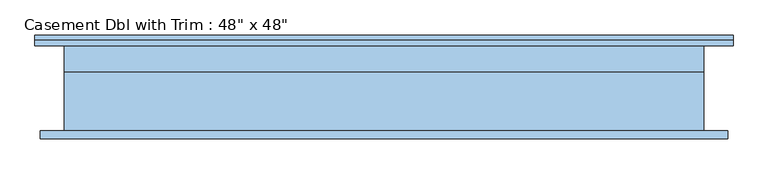
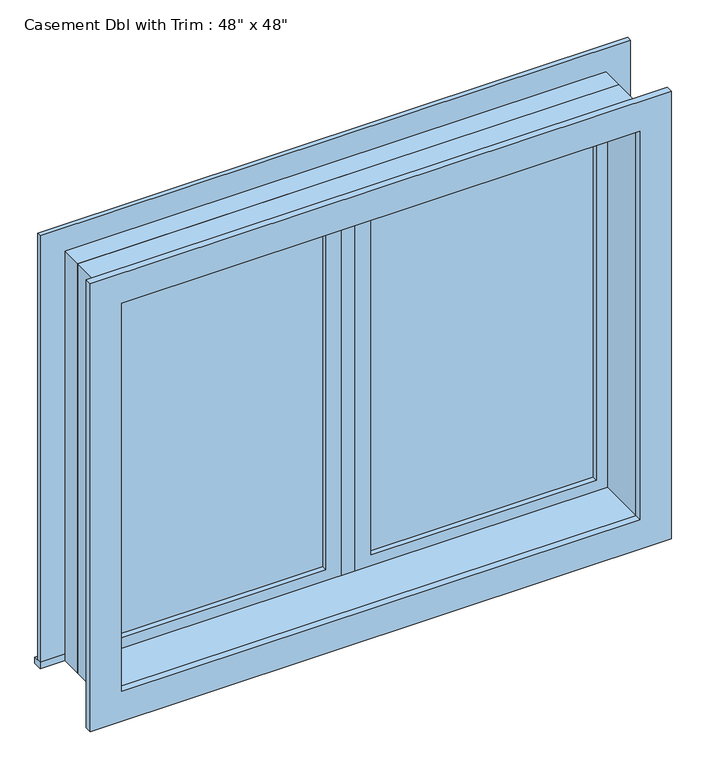
"""IFC4 building model written with IfcOpenShell, lengths in millimetres: window geometry."""

from ifc_helpers import new_model, si_unit, frame, origin, place, context, project, spatial, polyline, outline, extrude, source, transform, mapped, element, save


def window_03976a38(model_context):
    return source(origin(), model_context, "Body", "SweptSolid", [
        extrude(outline(polyline([(63.5, 85.725), (698.5, 85.725), (698.5, 73.025), (63.5, 73.025), (63.5, 85.725)])), frame((0.0, 0.0, 977.9), z_axis=(0.0, 0.0, 1.0), x_axis=(1.0, 0.0, 0.0)), (0.0, 0.0, 1.0), 1092.2),
        extrude(outline(polyline([(2114.55, 19.05), (933.45, 19.05), (933.45, 742.95), (2114.55, 742.95), (2114.55, 19.05)]), holes=[polyline([(2070.1, 63.5), (2070.1, 698.5), (977.9, 698.5), (977.9, 63.5), (2070.1, 63.5)])]), frame((0.0, 57.15, 0.0), z_axis=(0.0, 1.0, 0.0), x_axis=(0.0, 0.0, 1.0)), (0.0, 0.0, 1.0), 44.45),
        extrude(outline(polyline([(19.05, 57.15), (-19.05, 57.15), (-19.05, 120.65), (19.05, 120.65), (19.05, 57.15)])), frame((0.0, 0.0, 933.45), z_axis=(0.0, 0.0, 1.0), x_axis=(1.0, 0.0, 0.0)), (0.0, 0.0, 1.0), 1181.1),
        extrude(outline(polyline([(-831.85, 146.05), (831.85, 146.05), (831.85, 120.65), (-831.85, 120.65), (-831.85, 146.05)])), frame((0.0, 0.0, 914.4), z_axis=(0.0, 0.0, 1.0), x_axis=(1.0, 0.0, 0.0)), (0.0, 0.0, 1.0), 19.05),
        extrude(outline(polyline([(2114.55, -742.95), (2114.55, 742.95), (933.45, 742.95), (933.45, 831.85), (2203.45, 831.85), (2203.45, -831.85), (933.45, -831.85), (933.45, -742.95), (2114.55, -742.95)])), frame((0.0, 120.65, 0.0), z_axis=(0.0, 1.0, 0.0), x_axis=(0.0, 0.0, 1.0)), (0.0, 0.0, 1.0), 12.7),
        extrude(outline(polyline([(2190.75, 819.15), (2190.75, -819.15), (857.25, -819.15), (857.25, 819.15), (2190.75, 819.15)]), holes=[polyline([(2101.85, 730.25), (946.15, 730.25), (946.15, -730.25), (2101.85, -730.25), (2101.85, 730.25)])]), frame((0.0, -101.6, 0.0), z_axis=(0.0, 1.0, 0.0), x_axis=(0.0, 0.0, 1.0)), (0.0, 0.0, 1.0), 19.05),
        extrude(outline(polyline([(-63.5, 73.025), (-698.5, 73.025), (-698.5, 85.725), (-63.5, 85.725), (-63.5, 73.025)])), frame((0.0, 0.0, 977.9), z_axis=(0.0, 0.0, 1.0), x_axis=(1.0, 0.0, 0.0)), (0.0, 0.0, 1.0), 1092.2),
        extrude(outline(polyline([(2114.55, -742.95), (933.45, -742.95), (933.45, -19.05), (2114.55, -19.05), (2114.55, -742.95)]), holes=[polyline([(2070.1, -698.5), (2070.1, -63.5), (977.9, -63.5), (977.9, -698.5), (2070.1, -698.5)])]), frame((0.0, 57.15, 0.0), z_axis=(0.0, 1.0, 0.0), x_axis=(0.0, 0.0, 1.0)), (0.0, 0.0, 1.0), 44.45),
        extrude(outline(polyline([(2133.6, -762.0), (914.4, -762.0), (914.4, 762.0), (2133.6, 762.0), (2133.6, -762.0)]), holes=[polyline([(2101.85, -730.25), (2101.85, 730.25), (946.15, 730.25), (946.15, -730.25), (2101.85, -730.25)])]), frame((0.0, -82.55, 0.0), z_axis=(0.0, 1.0, 0.0), x_axis=(0.0, 0.0, 1.0)), (0.0, 0.0, 1.0), 139.7),
        extrude(outline(polyline([(2133.6, 762.0), (2133.6, -762.0), (914.4, -762.0), (914.4, 762.0), (2133.6, 762.0)]), holes=[polyline([(2114.55, 742.95), (933.45, 742.95), (933.45, -742.95), (2114.55, -742.95), (2114.55, 742.95)])]), frame((0.0, 57.15, 0.0), z_axis=(0.0, 1.0, 0.0), x_axis=(0.0, 0.0, 1.0)), (0.0, 0.0, 1.0), 63.5),
    ])


if __name__ == "__main__":
    model = new_model("IFC4")
    model_context = context("Model", 3, world=origin())
    ifc_project = project(units=[si_unit("LENGTHUNIT", "METRE", prefix="MILLI")], contexts=[model_context])
    site = spatial("IfcSite", under=ifc_project)
    building = spatial("IfcBuilding", under=site)
    placement = place(None, origin())
    window_shape = window_03976a38(model_context)
    element("IfcWindow", 1, ObjectType="Casement Dbl with Trim : 48\" x 48\"", at=placement, inside=building, context=model_context, shape_type="MappedRepresentation", body=[
        mapped(window_shape, transform((0.0, 0.0, 0.0), x_axis=(1.0, 0.0, 0.0), y_axis=(0.0, 1.0, 0.0), z_axis=(0.0, 0.0, 1.0))),
    ])
    save(model, "model.ifc")

# Revit data of these elements
# Type "Casement Dbl with Trim : 48\" x 48\""
#   Type Mark = "10"
#   Construction Type Id = "GSP4R"
#   Assembly Code = "B2020100"
#   Analytic Construction = "1/8 in Pilkington single glazing"
#   Visual Light Transmittance = 0.9
#   Solar Heat Gain Coefficient = 0.78
#   Heat Transfer Coefficient (U) = 0.6496 BTU/(h·ft²·°F)
#   Height = 4' - 0"
#   Default Sill Height = 3' - 0"
#   Trim Projection - Ext. = 0' - 0 1/2"
#   Trim Projection - Int. = 0' - 0 3/4"
#   Trim Width - Exterior = 0' - 3 1/2"
#   Trim Width - Interior = 0' - 3 1/2"
#   Width = 5' - 0"
#   Window Inset = 0' - 0 3/4"
#   Define Thermal Properties by = 1
#   Glass Pane Material = Glass
#   Sash Material = Sash
#   Trim Exterior Material = Trim
#   Trim Interior Material = Trim
#   Wall Closure = (empty or 0)
# Element 1 (IfcWindow, "Casement Dbl with Trim : 48\" x 48\"")
#   Materials on its faces: "Sash", "Trim", "Glass"
# Materials
#   "Glass": class "Glass", colour RGB 0 128 192, transparency 0.75, Description = "Soda Lime Glass", Cost = 0
#   "Sash": class "Wood", colour RGB 224 178 126, transparency 0
#   "Trim": class "Wood", colour RGB 224 178 126, transparency 0
